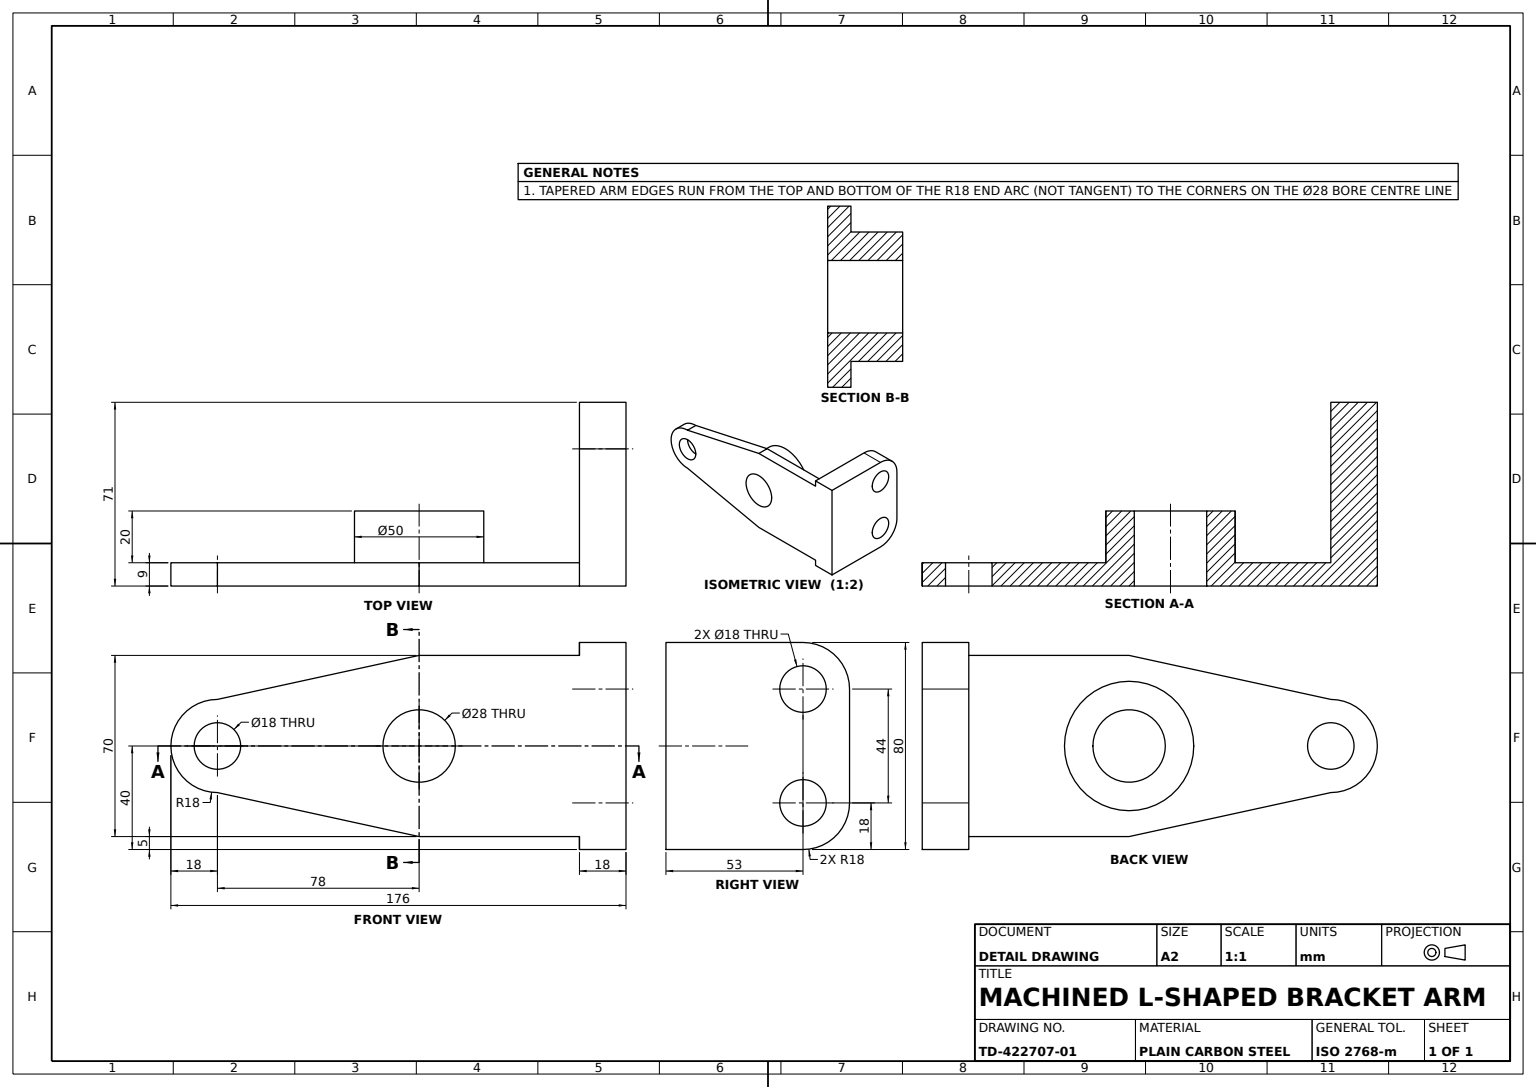
from build123d import *

# Parameters (mm, degrees)
BASE_PLATE_DEPTH              = 9
END_HOLE_18_SKETCH_R          = 9
END_HOLE_18_DEPTH             = 9
PIVOT_BOSS_50_SKETCH_R        = 25
PIVOT_BOSS_50_DEPTH           = 20
PIVOT_BORE_28_SKETCH_R        = 14
PIVOT_BORE_28_DEPTH           = 126.227792442
MOUNTING_BLOCK_DEPTH          = 18
MOUNTING_HOLES_2X_18_SKETCH_R = 9
MOUNTING_HOLES_2X_18_DEPTH    = 18


with BuildPart() as part:
    # Base Plate Profile Sketch → Base Plate (new body)
    with BuildSketch(Plane.XY):
        with BuildLine():
            Line((-78, 53), (0, 70))
            Line((0, 70), (69.753049234, 70))
            ThreePointArc((69.753049234, 70), (75.45392636, 71.316678554), (80, 75))
            Line((80, 75), (80, -5))
            ThreePointArc((80, -5), (75.45392636, -1.316678554), (69.753049234, 0))
            Line((69.753049234, 0), (0, 0))
            Line((0, 0), (-78, 17))
            ThreePointArc((-78, 17), (-96, 35), (-78, 53))
        make_face()
    extrude(amount=BASE_PLATE_DEPTH)

    # End Hole Ø18 Sketch → End Hole Ø18 (cut)
    with BuildSketch(Plane(origin=(0, 0, 0), x_dir=(-1, 0, 0), z_dir=(0, 0, -1))):
        with Locations((78, 35)):
            Circle(END_HOLE_18_SKETCH_R)
    extrude(amount=-END_HOLE_18_DEPTH, mode=Mode.SUBTRACT)

    # Pivot Boss Ø50 Sketch → Pivot Boss Ø50 (add)
    with BuildSketch(Plane(origin=(0, 0, 0), x_dir=(-1, 0, 0), z_dir=(0, 0, -1))):
        with Locations(Location((0, 35, 0), (0, 0, 180))):
            Circle(PIVOT_BOSS_50_SKETCH_R)
    extrude(amount=PIVOT_BOSS_50_DEPTH)

    # Pivot Bore Ø28 Sketch → Pivot Bore Ø28 (cut, through all)
    with BuildSketch(Plane(origin=(0, 0, -20), x_dir=(-1, 0, 0), z_dir=(0, 0, -1))):
        with Locations((0, 35)):
            Circle(PIVOT_BORE_28_SKETCH_R)
    extrude(amount=-PIVOT_BORE_28_DEPTH, mode=Mode.SUBTRACT)

    # Mounting Block Sketch → Mounting Block (add)
    with BuildSketch(Plane(origin=(80, 0, 0), x_dir=(0, 0, -1), z_dir=(1, 0, 0))):
        with BuildLine():
            Line((-9, 75), (44, 75))
            ThreePointArc((44, 75), (56.727922061, 69.727922061), (62, 57))
            Line((62, 57), (62, 13))
            ThreePointArc((62, 13), (56.727922061, 0.272077939), (44, -5))
            Line((44, -5), (-9, -5))
            Line((-9, -5), (-9, 75))
        make_face()
    extrude(amount=-MOUNTING_BLOCK_DEPTH)

    # Mounting Holes 2xØ18 Sketch → Mounting Holes 2xØ18 (cut)
    with BuildSketch(Plane(origin=(80, 0, 0), x_dir=(0, 0, -1), z_dir=(1, 0, 0))):
        with Locations((44, 57)):
            Circle(MOUNTING_HOLES_2X_18_SKETCH_R)
        with Locations((44, 13)):
            Circle(MOUNTING_HOLES_2X_18_SKETCH_R)
    extrude(amount=-MOUNTING_HOLES_2X_18_DEPTH, mode=Mode.SUBTRACT)


solid = part.part
